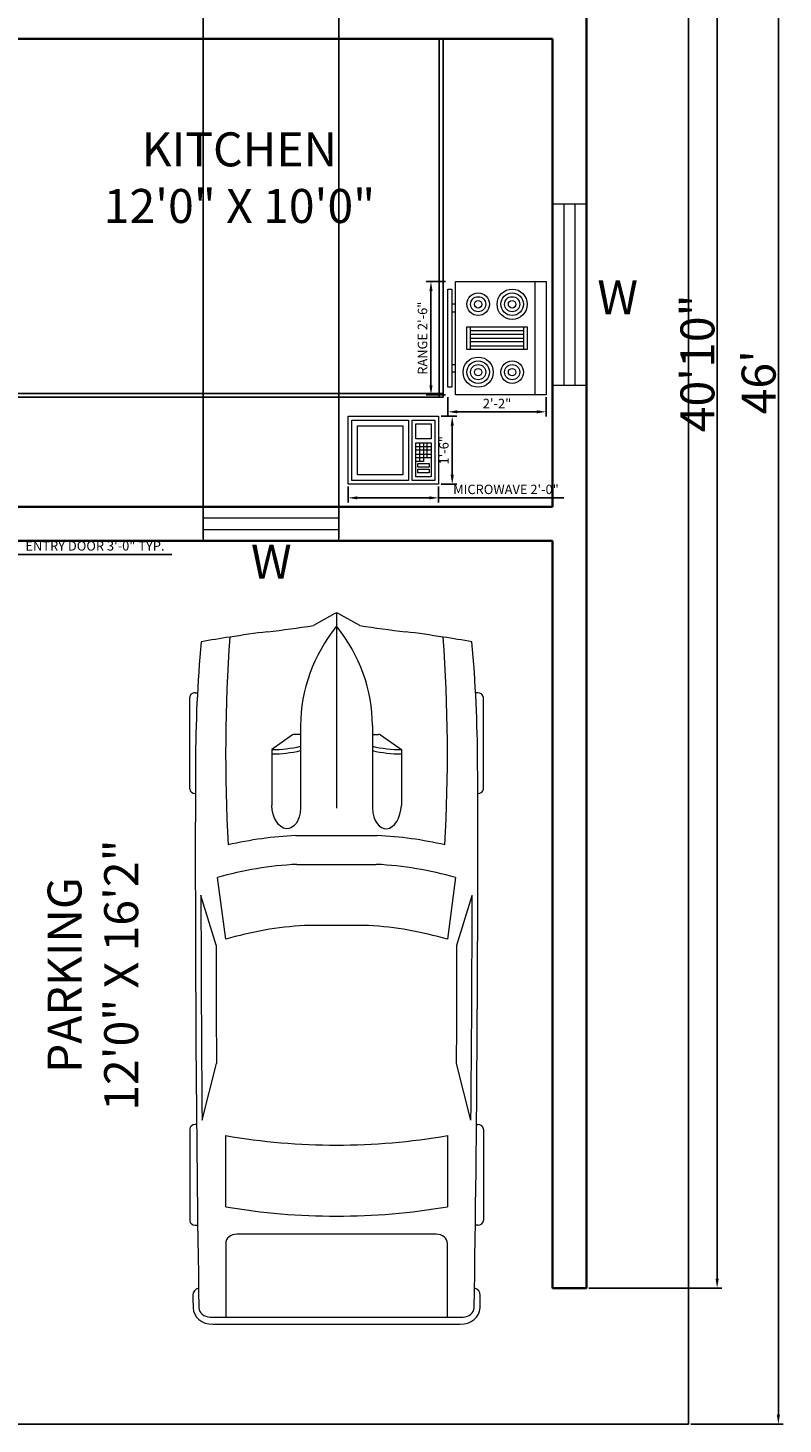
# Model space of a CAD drawing. Units: inches. Extents: x 1868 to 2413, y 1522 to 2138.
# Tile 3 of 4: x 2207 to 2408, y 1553 to 1923. Entities that reach past the tile are written whole.
import ezdxf

# ---------------------------------------------------------------- set-up
doc = ezdxf.new("R2010")
doc.units = ezdxf.units.IN
for name, color, linetype, lineweight in [('A-ANNO-DIMS', 2, 'Continuous', 18), ('A-ANNO-TEXT', 7, 'Continuous', 18), ('A-AREA-IDEN', 7, 'Continuous', 25), ('A-EQPM', 8, 'Continuous', 18), ('A-EQPM-VEHI', 9, 'Continuous', 13), ('A-FLOR-CASE', 8, 'Continuous', 25), ('A-GLAZ', 4, 'Continuous', 18), ('A-WALL', 7, 'Continuous', 35), ('C-PROP', 7, 'Continuous', 25)]:
    doc.layers.add(name, color=color, linetype=linetype, lineweight=lineweight)
doc.styles.get("Standard").update_dxf_attribs({"font": 'arial.ttf'})
doc.dimstyles.new('ISO-25', dxfattribs={"dimtxt": 2.5, "dimasz": 2.5, "dimexe": 1.25, "dimexo": 0.625, "dimtad": 1, "dimdec": 0, "dimlunit": 3, "dimtxsty": 'Standard', "dimcen": 2.5, "dimadec": 0, "dimazin": 0, "dimtfac": 1, "dimtdec": 0, "dimtmove": 0, "dimatfit": 3, "dimfxl": 1, "dimarcsym": 0})

# ---------------------------------------------------------------- blocks, each defined once
blk = doc.blocks.new('Range-Oven - 30 in top')
for p, q in [((0, -3), (30, -3)), ((12, -6), (18, -6)), ((13, -20), (13, -6)), ((14, -6), (14, -20)), ((15, -20), (15, -6)), ((16, -6), (16, -20)), ((17, -20), (17, -6)), ((18, -20), (12, -20)), ((6, -24), (6, -25)), ((8, -25), (8, -24)), ((22, -25), (22, -24)), ((24, -24), (24, -25))]:
    blk.add_line(p, q)
for points in [[(0, -24), (0, 0), (30, 0), (30, -24)], [(12, -21), (12, -5), (18, -5), (18, -21)], [(2, -26), (2, -25), (28, -25), (28, -26)]]:
    blk.add_lwpolyline(points, close=True)
for centre, radius in [((6, -9), 4), ((6, -9), 3), ((6, -9), 2), ((24, -9), 3), ((24, -9), 2), ((6, -9), 1), ((24, -9), 1), ((24, -18), 4), ((6, -18), 3), ((6, -18), 2), ((6, -18), 1), ((24, -18), 3), ((24, -18), 2), ((24, -18), 1)]:
    blk.add_circle(centre, radius)
blk = doc.blocks.new('Microwave')
for p, q in [((18, 10), (22, 10)), ((22, 9), (18, 9)), ((18, 8), (22, 8)), ((19, 7), (19, 11)), ((20, 11), (20, 7)), ((21, 7), (21, 11)), ((22, 7), (18, 7)), ((20, 6), (18, 6)), ((19, 6), (19, 7)), ((20, 7), (20, 6))]:
    blk.add_line(p, q)
for points in [[(0, 0), (0, 18), (24, 18), (24, 0)], [(1, 1), (1, 17), (16, 17), (16, 1)], [(2.5, 2.5), (2.5, 15.5), (14.5, 15.5), (14.5, 2.5)], [(17, 1), (17, 17), (23, 17), (23, 1)], [(18, 12), (18, 16), (22, 16), (22, 12)], [(18, 2), (18, 11), (22, 11), (22, 2)], [(18.5, 4.5), (18.5, 5.5), (21.5, 5.5), (21.5, 4.5)], [(18.5, 3), (18.5, 4), (21.5, 4), (21.5, 3)]]:
    blk.add_lwpolyline(points, close=True)
blk = doc.blocks.new('*D12')
at = {"layer": 'A-ANNO-DIMS', "color": 0, "lineweight": -2, "transparency": 16777216}
for p, q in [((2383.08, 2104.95), (2407.51, 2104.95)), ((2406.26, 2102.45), (2406.26, 1555.45)), ((2383.08, 1552.95), (2407.51, 1552.95))]:
    blk.add_line(p, q, dxfattribs=at)
at = {"layer": 'A-ANNO-DIMS', "color": 0, "transparency": 16777216}
for points in [[(2405.84, 2102.45), (2406.68, 2102.45), (2406.26, 2104.95)], [(2405.84, 1555.45), (2406.68, 1555.45), (2406.26, 1552.95)]]:
    blk.add_solid(points, dxfattribs=at)
at = {"layer": 'Defpoints', "color": 0, "transparency": 16777216}
for p in [(2382.46, 2104.95), (2382.46, 1552.95), (2406.26, 1552.95)]:
    blk.add_point(p, dxfattribs=at)
at = {"layer": 'A-ANNO-DIMS', "color": 0, "transparency": 16777216, "insert": (2401.04, 1828.95), "char_height": 2.5, "attachment_point": 5, "rotation": 90}
blk.add_mtext("{\\H3.6x;46'}", dxfattribs=at)
blk = doc.blocks.new('*D14')
at = {"layer": 'A-ANNO-DIMS', "color": 0, "lineweight": -2, "transparency": 16777216}
for p, q in [((2356.08, 2078.95), (2391.3, 2078.95)), ((2390.05, 2076.45), (2390.05, 1591.45)), ((2356.08, 1588.95), (2391.3, 1588.95))]:
    blk.add_line(p, q, dxfattribs=at)
at = {"layer": 'A-ANNO-DIMS', "color": 0, "transparency": 16777216}
for points in [[(2389.63, 2076.45), (2390.46, 2076.45), (2390.05, 2078.95)], [(2389.63, 1591.45), (2390.46, 1591.45), (2390.05, 1588.95)]]:
    blk.add_solid(points, dxfattribs=at)
at = {"layer": 'Defpoints', "color": 0, "transparency": 16777216}
for p in [(2355.46, 2078.95), (2355.46, 1588.95), (2390.05, 1588.95)]:
    blk.add_point(p, dxfattribs=at)
at = {"layer": 'A-ANNO-DIMS', "color": 0, "transparency": 16777216, "insert": (2384.83, 1833.95), "char_height": 2.5, "attachment_point": 5, "rotation": 90}
blk.add_mtext('{\\H3.6x;40\'10"}', dxfattribs=at)
blk = doc.blocks.new('*U16')
for p, q in [((21.1, 37.41), (21.1, 36.83)), ((46.55, 38.89), (22.35, 38.89)), ((47.8, 37.39), (47.8, 37.41)), ((135.45, 37.07), (135.45, 37.41)), ((136.7, 38.89), (160.9, 38.89)), ((162.15, 37.41), (162.15, 36.77)), ((87.99, 31.87), (74.76, 35.92)), ((134.31, 35.6), (119.29, 31.78)), ((186.47, -33.5), (186.47, 33.5)), ((70.03, 31.54), (86.41, 29.35)), ((188.4, -32.76), (188.4, 32.76)), ((138.42, 29.35), (157.25, 29.35)), ((164.52, 26.39), (164.52, -26.39)), ((186.47, 29.35), (167.01, 29.35)), ((32.27, 11.63), (36.13, 17.17)), ((36.13, 17.17), (50.94, 17.17)), ((32.12, 9.51), (32.12, 11.15)), ((29.77, 9.51), (51.68, 9.51)), ((58.92, -10.77), (58.92, 10.77)), ((66.55, -10.53), (66.55, 10.53)), ((82.74, 8.5), (82.74, -8.5)), ((186.47, -10.53), (186.47, 10.53)), ((3.27, 6.13), (0.1, 0.41)), ((0, 0), (51.68, 0)), ((0.1, -0.41), (3.27, -6.13)), ((29.77, -9.51), (51.68, -9.51)), ((32.12, -9.51), (32.12, -11.15)), ((32.27, -11.63), (36.13, -17.17)), ((36.13, -17.17), (50.94, -17.17)), ((86.41, -29.35), (70.03, -31.54)), ((157.25, -29.35), (138.42, -29.35)), ((167.01, -29.35), (186.47, -29.35)), ((87.99, -31.87), (74.76, -35.92)), ((134.31, -35.6), (119.29, -31.78)), ((21.1, -37.41), (21.1, -36.83)), ((162.15, -37.41), (162.15, -36.77)), ((46.55, -38.89), (22.35, -38.89)), ((47.8, -37.39), (47.8, -37.41)), ((135.45, -37.07), (135.45, -37.41)), ((136.7, -38.89), (160.9, -38.89))]:
    blk.add_line(p, q)
for centre, major_axis, ratio, start_param, end_param in [((41.19, -490.86), (0, 528.23), 0.842304, 0.00281, 0.075598), ((22.35, 37.41), (0, -1.48), 0.842304, 3.141593, 4.712389), ((64.48, -10555.62), (0, 10593.03), 0.842304, -0.013397, 0.002797), ((46.55, 37.41), (0, 1.48), 0.842304, -1.570796, 0), ((136.7, 37.41), (0, -1.48), 0.842304, 3.141593, 4.712389), ((160.9, 37.41), (0, 1.48), 0.842304, -1.570796, 0), ((180.63, 35.84), (0, 2.22), 0.842304, -0.013017, 1.249894), ((64.48, -10556.36), (0, 10595.31), 0.842304, -0.013397, -0.013017), ((183.98, 32.76), (0, -5.25), 0.842304, 1.570796, 3.128196), ((266.03, -27.52), (0, 313.31), 0.842304, 1.367076, 1.39176), ((64.48, -10555.62), (0, -10591.55), 0.842304, 3.133765, 3.140441), ((183.98, 33.5), (0, -2.96), 0.842304, 1.570796, 3.128196), ((37.47, -593.96), (0, -623.33), 0.842304, 3.096046, 3.200911), ((135.29, 5.39), (0, 81.77), 0.842304, 1.245306, 1.50788), ((95.79, -3666.35), (0, -3698.24), 0.842304, 3.134049, 3.144098), ((259.18, -27.52), (0, -305.3), 0.842304, 4.528606, 4.561838), ((134.4, 5.39), (0, -89.78), 0.842304, 4.449482, 4.652344), ((149.6, 2.8), (0, -79.58), 0.842304, 4.372215, 4.640744), ((17.08, 0), (0, 147.02), 0.842304, 4.511394, 4.913384), ((35.91, 0), (0, 147.02), 0.842304, 4.511394, 4.913384), ((167.01, 26.39), (0, 2.96), 0.842304, 0, 1.570796), ((-204.49, 52.4), (0, -250.96), 0.842304, 1.385369, 1.434372), ((13.04, 17.01), (0, 27.42), 0.842304, 4.435146, 4.718221), ((14.2, 17.01), (0, 27.42), 0.842304, 4.435146, 4.718221), ((50.79, 13.34), (6.34, -0.36), 0.603834, -1.395552, 1.581315), ((32.75, 11.15), (0, 0.74), 0.842304, 0.879714, 1.570796), ((29.77, -46.66), (0, 56.17), 0.842304, 0, 0.590319), ((0.62, 0), (0, -0.74), 0.842304, 4.131459, 5.293319), ((29.77, 46.66), (0, 56.17), 0.842304, 2.551274, 3.141593), ((-204.49, -52.4), (0, 250.96), 0.842304, -1.434372, -1.385369), ((13.04, -17.01), (0, -27.42), 0.842304, 1.564964, 1.848039), ((14.2, -17.01), (0, -27.42), 0.842304, 1.564964, 1.848039), ((134.4, -5.39), (0, -89.78), 0.842304, -1.510751, -1.307889), ((135.29, -5.39), (0, -81.77), 0.842304, -1.50788, -1.245306), ((149.6, -2.8), (0, -79.58), 0.842304, -1.499151, -1.230623), ((32.75, -11.15), (0, -0.74), 0.842304, 4.712389, 5.403472), ((259.18, 27.52), (0, 305.3), 0.842304, 1.721348, 1.754579), ((266.03, 27.52), (0, 313.31), 0.842304, 1.749832, 1.774517), ((37.47, 593.96), (0, -623.33), 0.842304, -0.059319, 0.045547), ((167.01, -26.39), (0, -2.96), 0.842304, 4.712389, 6.283185), ((95.79, 3666.35), (0, -3698.24), 0.842304, -0.002505, 0.007544), ((183.98, -32.76), (0, -5.25), 0.842304, 0.013397, 1.570796), ((41.19, 490.86), (0, -528.23), 0.842304, -0.075598, -0.00281), ((64.48, 10555.62), (0, 10593.03), 0.842304, 3.138796, 3.15499), ((64.48, 10555.62), (0, -10591.55), 0.842304, 0.001152, 0.007828), ((180.63, -35.84), (0, -2.22), 0.842304, -1.249894, 0.013017), ((183.98, -33.5), (0, 2.96), 0.842304, 3.15499, 4.712389), ((22.35, -37.41), (0, 1.48), 0.842304, 1.570796, 3.141593), ((46.55, -37.41), (0, -1.48), 0.842304, 0, 1.570796), ((136.7, -37.41), (0, -1.48), 0.842304, -1.570796, 0), ((160.9, -37.41), (0, 1.48), 0.842304, 3.141593, 4.712389), ((64.48, 10556.36), (0, 10595.31), 0.842304, 3.15461, 3.15499)]:
    blk.add_ellipse(centre, major_axis=major_axis, ratio=ratio, start_param=start_param, end_param=end_param)
at = {"extrusion": (0, 0, -1)}
blk.add_ellipse((50.79, -13.34), major_axis=(6.34, 0.36), ratio=0.603834, start_param=-1.395552, end_param=1.581315, dxfattribs=at)
blk = doc.blocks.new('WIN-48IN')
for p, q in [((0, 48), (0, 0)), ((9, 48), (0, 48)), ((3, 48), (3, 0)), ((6, 0), (6, 48)), ((9, 0), (9, 48)), ((0, 0), (9, 0))]:
    blk.add_line(p, q)
blk = doc.blocks.new('*D32')
at = {"layer": 'A-ANNO-DIMS', "color": 0, "lineweight": -2, "transparency": 16777216}
for p, q in [((2166.46, 1778.58), (2166.46, 1784.6)), ((2168.96, 1783.35), (2199.96, 1783.35)), ((2202.46, 1778.58), (2202.46, 1784.6)), ((2202.46, 1783.35), (2245.57, 1783.35))]:
    blk.add_line(p, q, dxfattribs=at)
at = {"layer": 'A-ANNO-DIMS', "color": 0, "transparency": 16777216}
for points in [[(2168.96, 1783.77), (2168.96, 1782.93), (2166.46, 1783.35)], [(2199.96, 1783.77), (2199.96, 1782.93), (2202.46, 1783.35)]]:
    blk.add_solid(points, dxfattribs=at)
at = {"layer": 'Defpoints', "color": 0, "transparency": 16777216}
for p in [(2202.46, 1783.35), (2166.46, 1777.95), (2202.46, 1777.95)]:
    blk.add_point(p, dxfattribs=at)
at = {"layer": 'A-ANNO-DIMS', "color": 0, "transparency": 16777216, "insert": (2225.26, 1785.27), "char_height": 2.5, "attachment_point": 5}
blk.add_mtext('ENTRY DOOR 3\'-0" TYP.', dxfattribs=at)
blk = doc.blocks.new('*D44')
at = {"layer": 'A-ANNO-DIMS', "color": 0, "lineweight": -2, "transparency": 16777216}
for p, q in [((2318.13, 1855.61), (2313, 1855.61)), ((2314.25, 1853.11), (2314.25, 1828.11)), ((2318.13, 1825.61), (2313, 1825.61))]:
    blk.add_line(p, q, dxfattribs=at)
at = {"layer": 'A-ANNO-DIMS', "color": 0, "transparency": 16777216}
for points in [[(2313.83, 1853.11), (2314.67, 1853.11), (2314.25, 1855.61)], [(2313.83, 1828.11), (2314.67, 1828.11), (2314.25, 1825.61)]]:
    blk.add_solid(points, dxfattribs=at)
at = {"layer": 'Defpoints', "color": 0, "transparency": 16777216}
for p in [(2318.75, 1855.61), (2314.25, 1825.61), (2318.75, 1825.61)]:
    blk.add_point(p, dxfattribs=at)
at = {"layer": 'A-ANNO-DIMS', "color": 0, "transparency": 16777216, "insert": (2312.33, 1840.61), "char_height": 2.5, "attachment_point": 5, "rotation": 90}
blk.add_mtext('RANGE 2\'-6"', dxfattribs=at)
blk = doc.blocks.new('*D45')
at = {"layer": 'A-ANNO-DIMS', "color": 0, "lineweight": -2, "transparency": 16777216}
for p, q in [((2318.75, 1824.99), (2318.75, 1819.86)), ((2344.75, 1824.99), (2344.75, 1819.86)), ((2321.25, 1821.11), (2342.25, 1821.11))]:
    blk.add_line(p, q, dxfattribs=at)
at = {"layer": 'A-ANNO-DIMS', "color": 0, "transparency": 16777216}
for points in [[(2321.25, 1821.53), (2321.25, 1820.7), (2318.75, 1821.11)], [(2342.25, 1821.53), (2342.25, 1820.7), (2344.75, 1821.11)]]:
    blk.add_solid(points, dxfattribs=at)
at = {"layer": 'Defpoints', "color": 0, "transparency": 16777216}
for p in [(2318.75, 1825.61), (2344.75, 1825.61), (2344.75, 1821.11)]:
    blk.add_point(p, dxfattribs=at)
at = {"layer": 'A-ANNO-DIMS', "color": 0, "transparency": 16777216, "insert": (2331.75, 1822.99), "char_height": 2.5, "attachment_point": 5}
blk.add_mtext('2\'-2"', dxfattribs=at)
blk = doc.blocks.new('*D46')
at = {"layer": 'A-ANNO-DIMS', "color": 0, "lineweight": -2, "transparency": 16777216}
for p, q in [((2292.28, 1801.29), (2292.28, 1797.07)), ((2316.28, 1801.29), (2316.28, 1797.07)), ((2294.78, 1798.32), (2313.78, 1798.32)), ((2316.28, 1798.32), (2349.46, 1798.32))]:
    blk.add_line(p, q, dxfattribs=at)
at = {"layer": 'A-ANNO-DIMS', "color": 0, "transparency": 16777216}
for points in [[(2294.78, 1798.73), (2294.78, 1797.9), (2292.28, 1798.32)], [(2313.78, 1798.73), (2313.78, 1797.9), (2316.28, 1798.32)]]:
    blk.add_solid(points, dxfattribs=at)
at = {"layer": 'Defpoints', "color": 0, "transparency": 16777216}
for p in [(2292.28, 1801.92), (2316.28, 1801.92), (2316.28, 1798.32)]:
    blk.add_point(p, dxfattribs=at)
at = {"layer": 'A-ANNO-DIMS', "color": 0, "transparency": 16777216, "insert": (2334.12, 1800.24), "char_height": 2.5, "attachment_point": 5}
blk.add_mtext('MICROWAVE 2\'-0"', dxfattribs=at)
blk = doc.blocks.new('*D47')
at = {"layer": 'A-ANNO-DIMS', "color": 0, "lineweight": -2, "transparency": 16777216}
for p, q in [((2316.91, 1819.92), (2321.13, 1819.92)), ((2319.88, 1804.42), (2319.88, 1817.42)), ((2316.91, 1801.92), (2321.13, 1801.92))]:
    blk.add_line(p, q, dxfattribs=at)
at = {"layer": 'A-ANNO-DIMS', "color": 0, "transparency": 16777216}
for points in [[(2319.46, 1817.42), (2320.3, 1817.42), (2319.88, 1819.92)], [(2319.46, 1804.42), (2320.3, 1804.42), (2319.88, 1801.92)]]:
    blk.add_solid(points, dxfattribs=at)
at = {"layer": 'Defpoints', "color": 0, "transparency": 16777216}
for p in [(2316.28, 1819.92), (2319.88, 1819.92), (2316.28, 1801.92)]:
    blk.add_point(p, dxfattribs=at)
at = {"layer": 'A-ANNO-DIMS', "color": 0, "transparency": 16777216, "insert": (2317.98, 1810.92), "char_height": 2.5, "attachment_point": 5, "rotation": 90}
blk.add_mtext('1\'-6"', dxfattribs=at)
blk = doc.blocks.new('*D56')
at = {"layer": 'A-ANNO-DIMS', "color": 0, "lineweight": -2, "transparency": 16777216}
for p, q in [((2253.87, 1787.58), (2253.87, 2135.38)), ((2256.37, 2134.13), (2287.37, 2134.13)), ((2289.87, 1787.58), (2289.87, 2135.38))]:
    blk.add_line(p, q, dxfattribs=at)
at = {"layer": 'A-ANNO-DIMS', "color": 0, "transparency": 16777216}
for points in [[(2256.37, 2134.54), (2256.37, 2133.71), (2253.87, 2134.13)], [(2287.37, 2134.54), (2287.37, 2133.71), (2289.87, 2134.13)]]:
    blk.add_solid(points, dxfattribs=at)
at = {"layer": 'Defpoints', "color": 0, "transparency": 16777216}
for p in [(2289.87, 2134.13), (2253.87, 1786.95), (2289.87, 1786.95)]:
    blk.add_point(p, dxfattribs=at)
at = {"layer": 'A-ANNO-DIMS', "color": 0, "transparency": 16777216, "insert": (2271.87, 2136.03), "char_height": 2.5, "attachment_point": 5}
blk.add_mtext('3\'-0"', dxfattribs=at)

msp = doc.modelspace()

# ---------------------------------------------------------------- linework, layer by layer
at = {"layer": 'A-FLOR-CASE'}
for p, q in [((2316.46, 1824.95), (2316.46, 1919.95)), ((2317.46, 1824.95), (2317.46, 1919.95)), ((2317.46, 1825.95), (2202.46, 1825.95)), ((2317.46, 1824.95), (2202.46, 1824.95))]:
    msp.add_line(p, q, dxfattribs=at)
at = {"layer": 'A-GLAZ'}
for p, q in [((2289.87, 1795.95), (2253.87, 1795.95)), ((2253.87, 1795.95), (2253.87, 1786.95)), ((2289.87, 1786.95), (2289.87, 1795.95)), ((2289.87, 1792.95), (2253.87, 1792.95)), ((2253.87, 1789.95), (2289.87, 1789.95)), ((2253.87, 1786.95), (2289.87, 1786.95))]:
    msp.add_line(p, q, dxfattribs=at)
at = {"layer": 'A-WALL'}
for p, q in [((2355.46, 1588.95), (2355.46, 2078.95)), ((2346.46, 1919.95), (2202.46, 1919.95)), ((2346.46, 1795.95), (2346.46, 1919.95)), ((2346.46, 1795.95), (2202.46, 1795.95)), ((2346.46, 1786.95), (2202.46, 1786.95)), ((2346.46, 1597.95), (2346.46, 1786.95)), ((2346.46, 1597.95), (2346.46, 1588.95)), ((2346.46, 1588.95), (2355.46, 1588.95))]:
    msp.add_line(p, q, dxfattribs=at)
at = {"layer": 'C-PROP'}
for p, q in [((2382.46, 1552.95), (2382.46, 2104.95)), ((1902.46, 1552.95), (2382.46, 1552.95))]:
    msp.add_line(p, q, dxfattribs=at)

# ---------------------------------------------------------------- block references
at = {"layer": 'A-EQPM', "rotation": 270}
msp.add_blockref('Range-Oven - 30 in top', (2344.75, 1855.61), dxfattribs=at)
at = {"layer": 'A-EQPM'}
msp.add_blockref('Microwave', (2292.28, 1801.92), dxfattribs=at)
at = {"layer": 'A-EQPM-VEHI', "rotation": 270}
msp.add_blockref('*U16', (2289.24, 1767.78), dxfattribs=at)
at = {"layer": 'A-GLAZ'}
msp.add_blockref('WIN-48IN', (2346.46, 1828.16), dxfattribs=at)

# ---------------------------------------------------------------- texts
at = {"layer": 'A-ANNO-TEXT', "char_height": 9, "attachment_point": 1}
for insert in [(2321.81, 1855.97), (2230.07, 1785.91)]:
    msp.add_mtext_dynamic_manual_height_columns('\\pxqc;W', width=83.7859, gutter_width=12.5, heights=[0], dxfattribs=dict(at, insert=insert))
at = {"layer": 'A-AREA-IDEN', "insert": (2217.3, 1895.14), "char_height": 9, "attachment_point": 1}
msp.add_mtext_dynamic_manual_height_columns('\\pxqc;KITCHEN\\P12\'0" X 10\'0"', width=92.4426, gutter_width=12.5, heights=[0], dxfattribs=at)
at = {"layer": 'A-AREA-IDEN', "insert": (2212.7, 1608.33), "char_height": 9, "attachment_point": 1, "rotation": 90}
msp.add_mtext_dynamic_manual_height_columns('\\pxqc;PARKING \\P12\'0" X 16\'2"', width=127.1139, gutter_width=12.5, heights=[0], dxfattribs=at)

# ---------------------------------------------------------------- dimensions: what is measured, and where the dimension line sits
at = {"layer": 'A-ANNO-DIMS'}
for base, p1, p2, picture, middle in [((2289.87, 2134.13), (2253.87, 1786.95), (2289.87, 1786.95), '*D56', (2271.87, 2136.03)), ((2344.75, 1821.11), (2318.75, 1825.61), (2344.75, 1825.61), '*D45', (2331.75, 1822.99))]:
    dim = msp.add_linear_dim(base=base, p1=p1, p2=p2, dimstyle='ISO-25', override={"dimdec": 1, "dimlfac": 1, "dimrnd": 0, "dimzin": 1, "dimdsep": 46, "dimlunit": 4, "dimfrac": 2}, dxfattribs=at)
    dim.commit()
    dim.dimension.update_dxf_attribs({"geometry": picture, "text_midpoint": middle})
for base, p1, p2, angle, text, override, picture, middle in [((2406.26, 1552.95), (2382.46, 2104.95), (2382.46, 1552.95), 90, "{\\H3.6x;46'}", {"dimclrd": 0, "dimclre": 0, "dimclrt": 0}, '*D12', (2401.04, 1828.95)), ((2390.05, 1588.95), (2355.46, 2078.95), (2355.46, 1588.95), 90, '{\\H3.6x;40\'10"}', {"dimclrd": 0, "dimclre": 0, "dimclrt": 0}, '*D14', (2384.83, 1833.95)), ((2314.25, 1825.61), (2318.75, 1855.61), (2318.75, 1825.61), 270, 'RANGE <>', {"dimdec": 1, "dimlfac": 1, "dimrnd": 0, "dimzin": 1, "dimdsep": 46, "dimlunit": 4, "dimfrac": 2}, '*D44', (2312.33, 1840.61))]:
    dim = msp.add_linear_dim(base=base, p1=p1, p2=p2, angle=angle, text=text, dimstyle='ISO-25', override=override, dxfattribs=at)
    dim.commit()
    dim.dimension.update_dxf_attribs({"geometry": picture, "text_midpoint": middle})
dim = msp.add_linear_dim(base=(2319.88, 1819.92), p1=(2316.28, 1801.92), p2=(2316.28, 1819.92), angle=90, dimstyle='ISO-25', override={"dimdec": 1, "dimlfac": 1, "dimrnd": 0, "dimzin": 1, "dimdsep": 46, "dimlunit": 4, "dimfrac": 2}, dxfattribs=at)
dim.commit()
dim.dimension.update_dxf_attribs({"geometry": '*D47', "text_midpoint": (2317.98, 1810.92)})
for base, p1, p2, text, picture, middle in [((2316.28, 1798.32), (2292.28, 1801.92), (2316.28, 1801.92), 'MICROWAVE <>', '*D46', (2334.12, 1800.24)), ((2202.46, 1783.35), (2166.46, 1777.95), (2202.46, 1777.95), 'ENTRY DOOR <> TYP.', '*D32', (2225.26, 1785.27))]:
    dim = msp.add_linear_dim(base=base, p1=p1, p2=p2, text=text, dimstyle='ISO-25', override={"dimdec": 1, "dimlfac": 1, "dimrnd": 0, "dimzin": 1, "dimdsep": 46, "dimlunit": 4, "dimfrac": 2}, dxfattribs=at)
    dim.commit()
    dim.dimension.update_dxf_attribs({"geometry": picture, "text_midpoint": middle})

doc.saveas('drawing.dxf')
